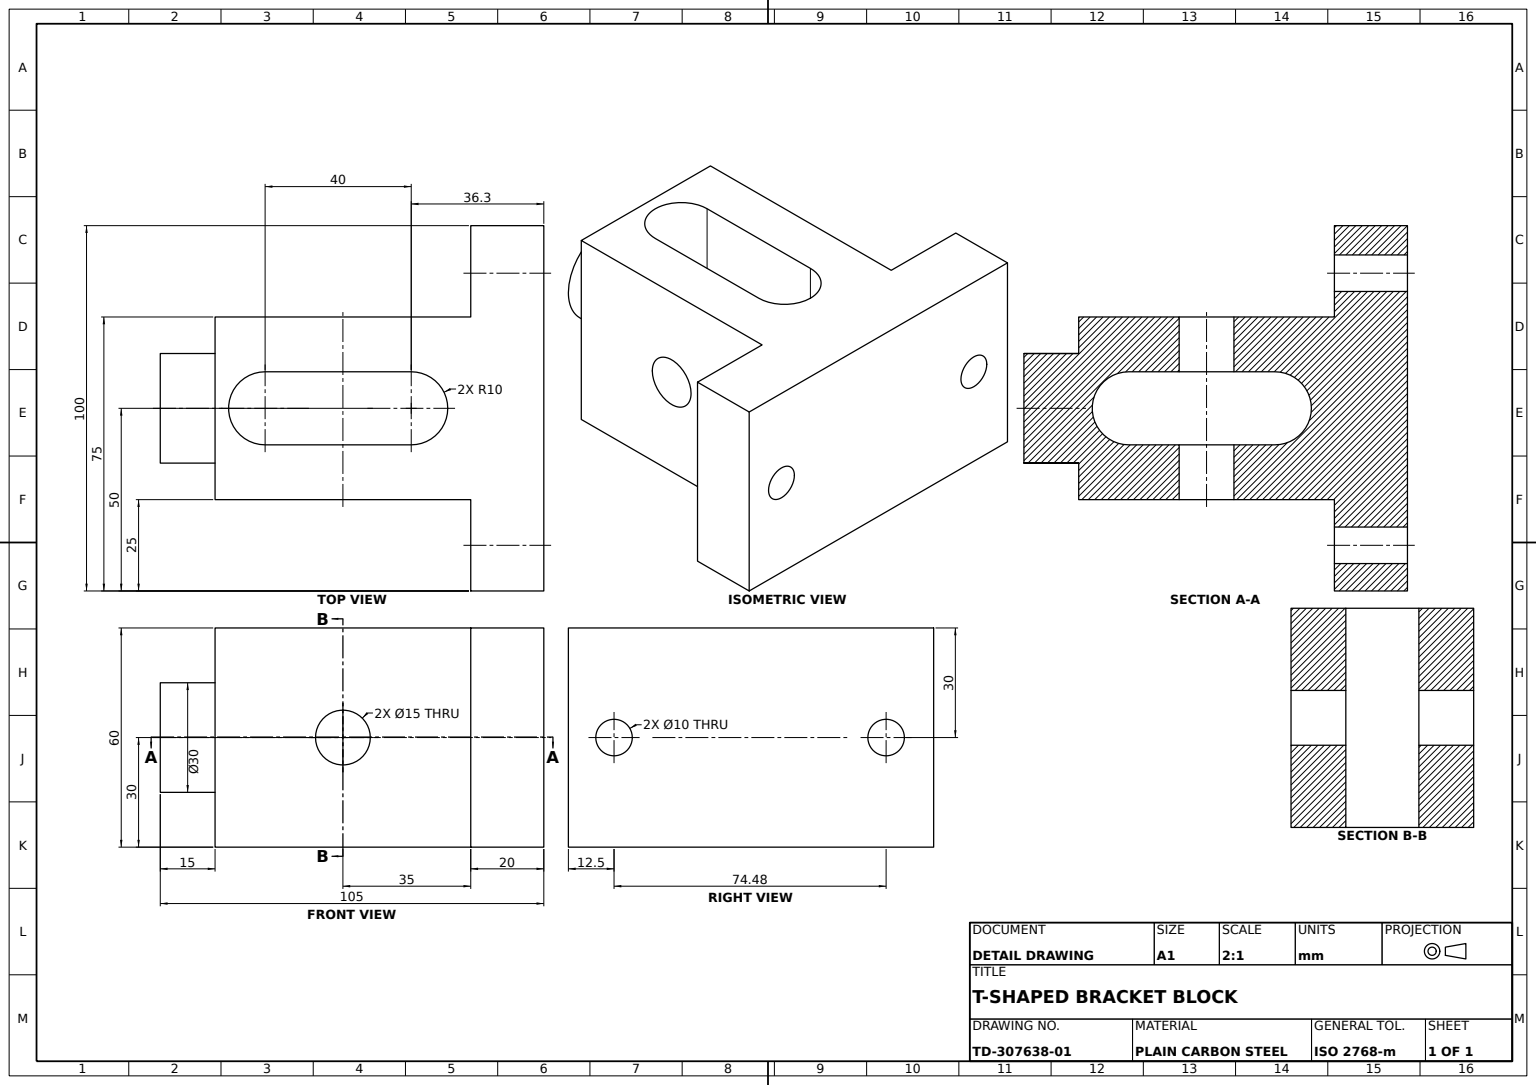
from build123d import *

# Parameters (mm, degrees)
BASE_PLATE_SKETCH_W      = 100
BASE_PLATE_SKETCH_H      = 60
BASE_PLATE_DEPTH         = 20
UPRIGHT_BLOCK_DEPTH      = 60
TOP_SLOT_DEPTH           = 60
NOTCH_SKETCH_R           = 5
NOTCH_CUT_DEPTH          = 20
CROSS_HOLE_A_15_SKETCH_R = 7.5
CROSS_HOLE_A_15_DEPTH    = 25
CROSS_START              = -25
CROSS_HOLE_B_15_SKETCH_R = 7.5
CROSS_HOLE_B_15_DEPTH    = 25
PIN_BOSS_30_SKETCH_R     = 15
PIN_BOSS_30_DEPTH        = 15


with BuildPart() as part:
    # Base Plate Sketch → Base Plate (new body)
    with BuildSketch(Plane.XY):
        with Locations((50, 30)):
            Rectangle(BASE_PLATE_SKETCH_W, BASE_PLATE_SKETCH_H)
    extrude(amount=BASE_PLATE_DEPTH)

    # Upright Block Sketch → Upright Block (add)
    with BuildSketch(Plane.XZ):
        Polygon((50, 20), (25, 20), (25, 90), (75, 90), (75, 20), align=None)
    extrude(amount=-UPRIGHT_BLOCK_DEPTH)

    # Top Slot Sketch → Top Slot (cut)
    with BuildSketch(Plane.XZ):
        with BuildLine():
            Line((40, 76.29728725), (40, 36.29728725))
            ThreePointArc((40, 36.29728725), (50, 26.29728725), (60, 36.29728725))
            Line((60, 36.29728725), (60, 76.29728725))
            ThreePointArc((60, 76.29728725), (50, 86.29728725), (40, 76.29728725))
        make_face()
    extrude(amount=-TOP_SLOT_DEPTH, mode=Mode.SUBTRACT)

    # Notch Sketch → Notch Cut (cut)
    with BuildSketch(Plane.XY.offset(20)):
        with Locations((87.5, 30)):
            Circle(NOTCH_SKETCH_R)
        with Locations((13.016158592, 30)):
            Circle(NOTCH_SKETCH_R)
    extrude(amount=-NOTCH_CUT_DEPTH, mode=Mode.SUBTRACT)

    # Cross Hole A Ø15 Sketch → Cross Hole A Ø15 (cut)
    with BuildSketch(Plane(origin=(75, 0, 0), x_dir=(0, 0, -1), z_dir=(1, 0, 0))):
        with Locations((-55, 30)):
            Circle(CROSS_HOLE_A_15_SKETCH_R)
    extrude(amount=-CROSS_HOLE_A_15_DEPTH, mode=Mode.SUBTRACT)

    # Cross Hole B Ø15 Sketch → Cross Hole B Ø15 (cut)
    with BuildSketch(Plane.ZY.offset(-25).offset(CROSS_START)):
        with Locations(Location((55, 30, 0), (0, 0, 180))):
            Circle(CROSS_HOLE_B_15_SKETCH_R)
    extrude(amount=CROSS_HOLE_B_15_DEPTH, mode=Mode.SUBTRACT)

    # Pin Boss Ø30 Sketch → Pin Boss Ø30 (add)
    with BuildSketch(Plane.XY.offset(90)):
        with Locations((50, 30)):
            Circle(PIN_BOSS_30_SKETCH_R)
    extrude(amount=PIN_BOSS_30_DEPTH)


solid = part.part
